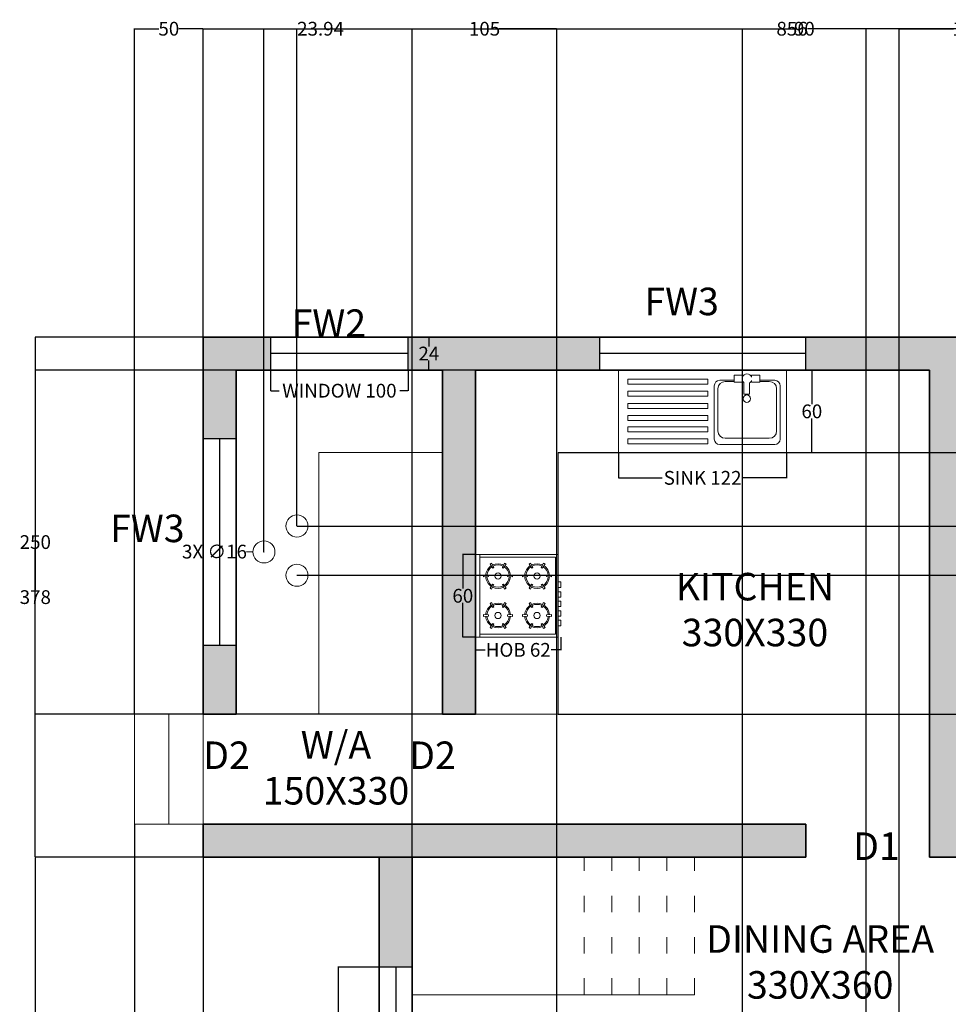
# Model space of a CAD drawing. Units: centimetres. Extents: x 1399 to 2860, y -110 to 1386.
# Tile 2 of 3: x 1399 to 2074, y 670 to 1386. Entities that reach past the tile are written whole.
import ezdxf

# ---------------------------------------------------------------- set-up
doc = ezdxf.new("R2010")
doc.units = ezdxf.units.CM
doc.header["$MEASUREMENT"] = 0
doc.linetypes.add('ACAD_ISO03W100', pattern=[30, 12, -18])
for name, color, linetype, lineweight in [('A-ANNO-DIMS', 2, 'Continuous', 18), ('A-ANNO-TEXT', 7, 'Continuous', 18), ('A-AREA-IDEN', 7, 'Continuous', 25), ('A-EQPM', 9, 'Continuous', 18), ('A-FLOR-CASE', 9, 'Continuous', 18), ('A-FLOR-FIXT', 9, 'Continuous', 18), ('A-FLOR-STRS', 7, 'Continuous', 18), ('A-FLOR-STRS-OVHD', 8, 'ACAD_ISO03W100', 18), ('A-GLAZ', 4, 'Continuous', 25), ('A-WALL', 7, 'Continuous', 35), ('A-WALL-PATT', 252, 'Continuous', 13)]:
    doc.layers.add(name, color=color, linetype=linetype, lineweight=lineweight)
doc.styles.get("Standard").update_dxf_attribs({"font": 'arial.ttf'})
doc.dimstyles.get("Standard").update_dxf_attribs({"dimtxt": 10, "dimasz": 0.18, "dimexe": 0.18, "dimexo": 0.0625, "dimgap": 0.09, "dimtad": 0, "dimtih": 1, "dimtoh": 1, "dimdec": 4, "dimzin": 0, "dimdsep": 46, "dimtxsty": 'Standard', "dimcen": 0.09, "dimadec": 0, "dimazin": 0, "dimtfac": 1, "dimtdec": 4, "dimtofl": 0, "dimtmove": 0, "dimatfit": 3, "dimfxl": 1, "dimtolj": 1, "dimtzin": 0, "dimarcsym": 0})

# ---------------------------------------------------------------- blocks, each defined once
blk = doc.blocks.new('w2')
blk.add_line((1776.97, 1807.89), (1676.97, 1807.89))
blk.add_lwpolyline([(1676.97, 1795.89), (1776.97, 1795.89), (1776.97, 1819.89), (1676.97, 1819.89)], close=True)
blk = doc.blocks.new('w3')
blk.add_line((1235.35, 1319.41), (1085.35, 1319.41))
blk.add_lwpolyline([(1085.35, 1307.41), (1235.35, 1307.41), (1235.35, 1331.41), (1085.35, 1331.41)], close=True)
blk = doc.blocks.new('A$C27DD639B')
for p, q in [((0, 0), (0, 450)), ((0, 450), (916.2, 450)), ((916.2, 0), (916.2, 450)), ((50.5, 372.3), (50.5, 400.1)), ((50.5, 400.1), (486.3, 400.1)), ((486.3, 400.1), (486.3, 372.3)), ((551.5, 394.1), (630.4, 394.1)), ((581.5, 388), (630.4, 388)), ((630.4, 383.4), (630.4, 422.8)), ((630.4, 422.8), (674.9, 422.8)), ((674.9, 383.4), (630.4, 383.4)), ((674.9, 422.8), (674.9, 411.1)), ((674.9, 394.1), (674.9, 383.4)), ((683, 318.7), (683, 382.1)), ((714.2, 379.9), (714.2, 318.7)), ((725.3, 411.7), (725.3, 422.8)), ((725.3, 422.8), (769.8, 422.8)), ((725.3, 383.4), (725.3, 393.5)), ((769.8, 383.4), (725.3, 383.4)), ((769.8, 422.8), (769.8, 383.4)), ((769.8, 394.1), (851.5, 394.1)), ((769.8, 388), (821.5, 388)), ((486.3, 372.3), (50.5, 372.3)), ((50.5, 307.4), (50.5, 335.2)), ((50.5, 335.2), (486.3, 335.2)), ((486.3, 335.2), (486.3, 307.4)), ((521.5, 74.1), (521.5, 364.1)), ((541.5, 118), (541.5, 348)), ((861.5, 348), (861.5, 118)), ((881.5, 364.1), (881.5, 74.1)), ((486.3, 307.4), (50.5, 307.4)), ((714.2, 318.7), (683, 318.7)), ((50.5, 240.3), (50.5, 268.1)), ((50.5, 268.1), (486.3, 268.1)), ((486.3, 240.3), (50.5, 240.3)), ((486.3, 268.1), (486.3, 240.3)), ((50.5, 175.4), (50.5, 203.2)), ((50.5, 203.2), (486.3, 203.2)), ((486.3, 175.4), (50.5, 175.4)), ((486.3, 203.2), (486.3, 175.4)), ((50.5, 112.8), (50.5, 140.6)), ((50.5, 140.6), (486.3, 140.6)), ((486.3, 112.8), (50.5, 112.8)), ((486.3, 140.6), (486.3, 112.8)), ((50.5, 48), (50.5, 75.8)), ((50.5, 75.8), (486.3, 75.8)), ((486.3, 75.8), (486.3, 48)), ((821.5, 78), (581.5, 78)), ((486.3, 48), (50.5, 48)), ((851.5, 44.1), (551.5, 44.1)), ((916.2, 0), (0, 0))]:
    blk.add_line(p, q)
blk.add_circle((699.5, 294.1), 20.1)
for centre, radius, start, end in [((700.2, 402.6), 26.7, 19.9093, 161.5199), ((551.5, 364.1), 30, 90, 180), ((581.5, 348), 40, 90, 180), ((700.2, 402.6), 26.7, 198.4801, 230.0288), ((700.2, 402.6), 26.7, 301.5638, 340.0907), ((821.5, 348), 40, 0, 90), ((851.5, 364.1), 30, 0, 90), ((581.5, 118), 40, 180, 270), ((821.5, 118), 40, 270, 0), ((551.5, 74.1), 30, 180, 270), ((851.5, 74.1), 30, 270, 0)]:
    blk.add_arc(centre, radius, start, end)
blk = doc.blocks.new('A$C756A3D80')
for p, q in [((600, 620), (0, 620)), ((0, 620), (0, 20)), ((0, 590), (600, 590)), ((20, 590), (20, 40)), ((580, 40), (580, 590)), ((600, 20), (600, 620)), ((69, 515.1), (62.3, 503.4)), ((62.3, 503.4), (94.8, 487.7)), ((98.8, 494.7), (69, 515.1)), ((163.4, 561.8), (149.9, 561.8)), ((149.9, 561.8), (152.6, 525.8)), ((152.6, 525.8), (160.7, 525.8)), ((160.7, 525.8), (163.4, 561.8)), ((244.3, 515.1), (214.5, 494.7)), ((218.6, 487.7), (251.1, 503.4)), ((251.1, 503.4), (244.3, 515.1)), ((355.7, 515.1), (348.9, 503.4)), ((348.9, 503.4), (381.4, 487.7)), ((385.5, 494.7), (355.7, 515.1)), ((450.1, 561.8), (436.6, 561.8)), ((436.6, 561.8), (439.3, 525.8)), ((439.3, 525.8), (447.4, 525.8)), ((447.4, 525.8), (450.1, 561.8)), ((531, 515.1), (501.2, 494.7)), ((505.2, 487.7), (537.7, 503.4)), ((537.7, 503.4), (531, 515.1)), ((94.8, 487.7), (98.8, 494.7)), ((214.5, 494.7), (218.6, 487.7)), ((381.4, 487.7), (385.5, 494.7)), ((501.2, 494.7), (505.2, 487.7)), ((94.8, 425.6), (62.3, 410)), ((62.3, 410), (69, 398.3)), ((69, 398.3), (98.8, 418.6)), ((98.8, 418.6), (94.8, 425.6)), ((152.6, 387.5), (149.9, 351.5)), ((160.7, 387.5), (152.6, 387.5)), ((163.4, 351.5), (160.7, 387.5)), ((218.6, 425.6), (214.5, 418.6)), ((214.5, 418.6), (244.3, 398.3)), ((251.1, 410), (218.6, 425.6)), ((244.3, 398.3), (251.1, 410)), ((381.4, 425.6), (348.9, 410)), ((348.9, 410), (355.7, 398.3)), ((355.7, 398.3), (385.5, 418.6)), ((385.5, 418.6), (381.4, 425.6)), ((439.3, 387.5), (436.6, 351.5)), ((447.4, 387.5), (439.3, 387.5)), ((450.1, 351.5), (447.4, 387.5)), ((505.2, 425.6), (501.2, 418.6)), ((501.2, 418.6), (531, 398.3)), ((537.7, 410), (505.2, 425.6)), ((531, 398.3), (537.7, 410)), ((149.9, 351.5), (163.4, 351.5)), ((436.6, 351.5), (450.1, 351.5)), ((69, 231.7), (62.3, 220)), ((62.3, 220), (94.8, 204.4)), ((98.8, 211.4), (69, 231.7)), ((163.4, 278.5), (149.9, 278.5)), ((149.9, 278.5), (152.6, 242.5)), ((152.6, 242.5), (160.7, 242.5)), ((160.7, 242.5), (163.4, 278.5)), ((244.3, 231.7), (214.5, 211.4)), ((218.6, 204.4), (251.1, 220)), ((251.1, 220), (244.3, 231.7)), ((355.7, 231.7), (348.9, 220)), ((348.9, 220), (381.4, 204.4)), ((385.5, 211.4), (355.7, 231.7)), ((450.1, 278.5), (436.6, 278.5)), ((436.6, 278.5), (439.3, 242.5)), ((439.3, 242.5), (447.4, 242.5)), ((447.4, 242.5), (450.1, 278.5)), ((531, 231.7), (501.2, 211.4)), ((505.2, 204.4), (537.7, 220)), ((537.7, 220), (531, 231.7)), ((94.8, 204.4), (98.8, 211.4)), ((214.5, 211.4), (218.6, 204.4)), ((381.4, 204.4), (385.5, 211.4)), ((501.2, 211.4), (505.2, 204.4)), ((94.8, 142.3), (62.3, 126.6)), ((62.3, 126.6), (69, 114.9)), ((69, 114.9), (98.8, 135.3)), ((98.8, 135.3), (94.8, 142.3)), ((152.6, 104.2), (149.9, 68.2)), ((160.7, 104.2), (152.6, 104.2)), ((163.4, 68.2), (160.7, 104.2)), ((218.6, 142.3), (214.5, 135.3)), ((214.5, 135.3), (244.3, 114.9)), ((251.1, 126.6), (218.6, 142.3)), ((244.3, 114.9), (251.1, 126.6)), ((381.4, 142.3), (348.9, 126.6)), ((348.9, 126.6), (355.7, 114.9)), ((355.7, 114.9), (385.5, 135.3)), ((385.5, 135.3), (381.4, 142.3)), ((439.3, 104.2), (436.6, 68.2)), ((447.4, 104.2), (439.3, 104.2)), ((450.1, 68.2), (447.4, 104.2)), ((505.2, 142.3), (501.2, 135.3)), ((501.2, 135.3), (531, 114.9)), ((537.7, 126.6), (505.2, 142.3)), ((531, 114.9), (537.7, 126.6)), ((0, 20), (600, 20)), ((20, 40), (580, 40)), ((81.8, 20), (121.8, 20)), ((81.8, 0), (81.8, 20)), ((121.8, 20), (121.8, 0)), ((149.9, 68.2), (163.4, 68.2)), ((151.3, 20), (191.3, 20)), ((151.3, 0), (151.3, 20)), ((191.3, 20), (191.3, 0)), ((221.6, 20), (261.6, 20)), ((221.6, 0), (221.6, 20)), ((261.6, 20), (261.6, 0)), ((289.3, 20), (329.3, 20)), ((289.3, 0), (289.3, 20)), ((329.3, 20), (329.3, 0)), ((361, 20), (401, 20)), ((361, 0), (361, 20)), ((401, 20), (401, 0)), ((436.6, 68.2), (450.1, 68.2)), ((121.8, 0), (81.8, 0)), ((191.3, 0), (151.3, 0)), ((261.6, 0), (221.6, 0)), ((329.3, 0), (289.3, 0)), ((401, 0), (361, 0))]:
    blk.add_line(p, q)
for centre in [(156.7, 456.7), (443.3, 456.7), (156.7, 173.3), (443.3, 173.3)]:
    blk.add_circle(centre, 22.6)
for centre, radius, start, end in [((156.7, 456.7), 90, 93.56902, 146.43098), ((156.7, 456.7), 81, 93.489, 146.511), ((156.7, 456.7), 81, 33.489, 86.511), ((156.7, 456.7), 90, 33.56902, 86.43098), ((443.3, 456.7), 90, 93.56902, 146.43098), ((443.3, 456.7), 81, 93.489, 146.511), ((443.3, 456.7), 81, 33.489, 86.511), ((443.3, 456.7), 90, 33.56902, 86.43098), ((156.7, 456.7), 90, 153.56902, 206.43098), ((156.7, 456.7), 81, 153.489, 206.511), ((156.7, 456.7), 81, 333.489, 26.511), ((156.7, 456.7), 90, 333.56902, 26.43098), ((443.3, 456.7), 90, 153.56902, 206.43098), ((443.3, 456.7), 81, 153.489, 206.511), ((443.3, 456.7), 81, 333.489, 26.511), ((443.3, 456.7), 90, 333.56902, 26.43098), ((156.7, 456.7), 90, 213.56902, 266.43098), ((156.7, 456.7), 81, 213.489, 266.511), ((156.7, 456.7), 81, 273.489, 326.511), ((156.7, 456.7), 90, 273.56902, 326.43098), ((443.3, 456.7), 90, 213.56902, 266.43098), ((443.3, 456.7), 81, 213.489, 266.511), ((443.3, 456.7), 81, 273.489, 326.511), ((443.3, 456.7), 90, 273.56902, 326.43098), ((156.7, 173.3), 90, 93.56902, 146.43098), ((156.7, 173.3), 81, 93.489, 146.511), ((156.7, 173.3), 81, 33.489, 86.511), ((156.7, 173.3), 90, 33.56902, 86.43098), ((443.3, 173.3), 90, 93.56902, 146.43098), ((443.3, 173.3), 81, 93.489, 146.511), ((443.3, 173.3), 81, 33.489, 86.511), ((443.3, 173.3), 90, 33.56902, 86.43098), ((156.7, 173.3), 90, 153.56902, 206.43098), ((156.7, 173.3), 81, 153.489, 206.511), ((156.7, 173.3), 81, 333.489, 26.511), ((156.7, 173.3), 90, 333.56902, 26.43098), ((443.3, 173.3), 90, 153.56902, 206.43098), ((443.3, 173.3), 81, 153.489, 206.511), ((443.3, 173.3), 81, 333.489, 26.511), ((443.3, 173.3), 90, 333.56902, 26.43098), ((156.7, 173.3), 90, 213.56902, 266.43098), ((156.7, 173.3), 81, 213.489, 266.511), ((156.7, 173.3), 81, 273.489, 326.511), ((156.7, 173.3), 90, 273.56902, 326.43098), ((443.3, 173.3), 90, 213.56902, 266.43098), ((443.3, 173.3), 81, 213.489, 266.511), ((443.3, 173.3), 81, 273.489, 326.511), ((443.3, 173.3), 90, 273.56902, 326.43098)]:
    blk.add_arc(centre, radius, start, end)
blk = doc.blocks.new('W4')
blk.add_line((1292.48, 2297.53), (1492.48, 2297.53))
blk.add_lwpolyline([(1292.48, 2285.53), (1492.48, 2285.53), (1492.48, 2309.53), (1292.48, 2309.53)], close=True)
blk = doc.blocks.new('*D19')
at = {"layer": 'A-ANNO-DIMS', "color": 0, "lineweight": -2, "transparency": 16777216}
for p, q in [((1581.8, 1130.95), (1581.8, 1115.83)), ((1681.8, 1130.95), (1681.8, 1115.83)), ((1581.98, 1116.01), (1587.89, 1116.01)), ((1681.62, 1116.01), (1675.72, 1116.01))]:
    blk.add_line(p, q, dxfattribs=at)
at = {"layer": 'A-ANNO-DIMS', "color": 0, "transparency": 16777216}
for points in [[(1581.98, 1116.04), (1581.98, 1115.98), (1581.8, 1116.01)], [(1681.62, 1116.04), (1681.62, 1115.98), (1681.8, 1116.01)]]:
    blk.add_solid(points, dxfattribs=at)
at = {"layer": 'Defpoints', "color": 0, "transparency": 16777216}
for p in [(1581.8, 1131.01), (1681.8, 1131.01), (1681.8, 1116.01)]:
    blk.add_point(p, dxfattribs=at)
at = {"layer": 'A-ANNO-DIMS', "color": 0, "transparency": 16777216, "insert": (1631.8, 1116.01), "char_height": 10, "attachment_point": 5}
blk.add_mtext('\\A1;WINDOW 100', dxfattribs=at)
blk = doc.blocks.new('*D20')
at = {"layer": 'A-ANNO-DIMS', "color": 0, "lineweight": -2, "transparency": 16777216}
for p, q in [((1681.86, 1155.01), (1696.98, 1155.01)), ((1696.8, 1154.83), (1696.8, 1148.12)), ((1696.8, 1131.19), (1696.8, 1137.9)), ((1681.86, 1131.01), (1696.98, 1131.01))]:
    blk.add_line(p, q, dxfattribs=at)
at = {"layer": 'A-ANNO-DIMS', "color": 0, "transparency": 16777216}
for points in [[(1696.77, 1154.83), (1696.83, 1154.83), (1696.8, 1155.01)], [(1696.77, 1131.19), (1696.83, 1131.19), (1696.8, 1131.01)]]:
    blk.add_solid(points, dxfattribs=at)
at = {"layer": 'Defpoints', "color": 0, "transparency": 16777216}
for p in [(1681.8, 1155.01), (1696.8, 1155.01), (1681.8, 1131.01)]:
    blk.add_point(p, dxfattribs=at)
at = {"layer": 'A-ANNO-DIMS', "color": 0, "transparency": 16777216, "insert": (1696.8, 1143.01), "char_height": 10, "attachment_point": 5}
blk.add_mtext('\\A1;24', dxfattribs=at)
blk = doc.blocks.new('*D21')
at = {"layer": 'A-ANNO-DIMS', "color": 0, "lineweight": -2, "transparency": 16777216}
for p, q in [((1660.74, 697.01), (1630.62, 697.01)), ((1630.8, 696.83), (1630.8, 602.27)), ((1630.8, 497.19), (1630.8, 591.75)), ((1660.74, 497.01), (1630.62, 497.01))]:
    blk.add_line(p, q, dxfattribs=at)
at = {"layer": 'A-ANNO-DIMS', "color": 0, "transparency": 16777216}
for points in [[(1630.77, 696.83), (1630.83, 696.83), (1630.8, 697.01)], [(1630.77, 497.19), (1630.83, 497.19), (1630.8, 497.01)]]:
    blk.add_solid(points, dxfattribs=at)
at = {"layer": 'Defpoints', "color": 0, "transparency": 16777216}
for p in [(1660.8, 697.01), (1630.8, 497.01), (1660.8, 497.01)]:
    blk.add_point(p, dxfattribs=at)
at = {"layer": 'A-ANNO-DIMS', "color": 0, "transparency": 16777216, "insert": (1630.8, 597.01), "char_height": 10, "attachment_point": 5}
blk.add_mtext('\\A1;WINDOW 200', dxfattribs=at)
blk = doc.blocks.new('*D33')
at = {"layer": 'A-ANNO-DIMS', "color": 0, "lineweight": -2, "transparency": 16777216}
for p, q in [((1834.73, 1070.95), (1834.73, 1052.51)), ((1956.88, 1070.95), (1956.88, 1052.51)), ((1834.91, 1052.69), (1866.5, 1052.69)), ((1956.7, 1052.69), (1925.11, 1052.69))]:
    blk.add_line(p, q, dxfattribs=at)
at = {"layer": 'A-ANNO-DIMS', "color": 0, "transparency": 16777216}
for points in [[(1834.91, 1052.72), (1834.91, 1052.66), (1834.73, 1052.69)], [(1956.7, 1052.72), (1956.7, 1052.66), (1956.88, 1052.69)]]:
    blk.add_solid(points, dxfattribs=at)
at = {"layer": 'Defpoints', "color": 0, "transparency": 16777216}
for p in [(1834.73, 1071.01), (1956.88, 1071.01), (1956.88, 1052.69)]:
    blk.add_point(p, dxfattribs=at)
at = {"layer": 'A-ANNO-DIMS', "color": 0, "transparency": 16777216, "insert": (1895.8, 1052.69), "char_height": 10, "attachment_point": 5}
blk.add_mtext('\\A1;SINK 122', dxfattribs=at)
blk = doc.blocks.new('*D34')
at = {"layer": 'A-ANNO-DIMS', "color": 0, "lineweight": -2, "transparency": 16777216}
for p, q in [((1956.94, 1131.01), (1975.38, 1131.01)), ((1975.2, 1130.83), (1975.2, 1106.21)), ((1975.2, 1071.19), (1975.2, 1095.81)), ((1956.94, 1071.01), (1975.38, 1071.01))]:
    blk.add_line(p, q, dxfattribs=at)
at = {"layer": 'A-ANNO-DIMS', "color": 0, "transparency": 16777216}
for points in [[(1975.17, 1130.83), (1975.23, 1130.83), (1975.2, 1131.01)], [(1975.17, 1071.19), (1975.23, 1071.19), (1975.2, 1071.01)]]:
    blk.add_solid(points, dxfattribs=at)
at = {"layer": 'Defpoints', "color": 0, "transparency": 16777216}
for p in [(1956.88, 1131.01), (1975.2, 1131.01), (1956.88, 1071.01)]:
    blk.add_point(p, dxfattribs=at)
at = {"layer": 'A-ANNO-DIMS', "color": 0, "transparency": 16777216, "insert": (1975.2, 1101.01), "char_height": 10, "attachment_point": 5}
blk.add_mtext('\\A1;60', dxfattribs=at)
blk = doc.blocks.new('*D35')
at = {"layer": 'A-ANNO-DIMS', "color": 0, "lineweight": -2, "transparency": 16777216}
for p, q in [((1730.8, 936.91), (1730.8, 927.5)), ((1792.8, 936.91), (1792.8, 927.5)), ((1730.98, 927.68), (1737.79, 927.68)), ((1792.62, 927.68), (1785.81, 927.68))]:
    blk.add_line(p, q, dxfattribs=at)
at = {"layer": 'A-ANNO-DIMS', "color": 0, "transparency": 16777216}
for points in [[(1730.98, 927.71), (1730.98, 927.65), (1730.8, 927.68)], [(1792.62, 927.71), (1792.62, 927.65), (1792.8, 927.68)]]:
    blk.add_solid(points, dxfattribs=at)
at = {"layer": 'Defpoints', "color": 0, "transparency": 16777216}
for p in [(1730.8, 936.98), (1792.8, 936.98), (1730.8, 927.68)]:
    blk.add_point(p, dxfattribs=at)
at = {"layer": 'A-ANNO-DIMS', "color": 0, "transparency": 16777216, "insert": (1761.8, 927.68), "char_height": 10, "attachment_point": 5}
blk.add_mtext('\\A1;HOB 62', dxfattribs=at)
blk = doc.blocks.new('*D36')
at = {"layer": 'A-ANNO-DIMS', "color": 0, "lineweight": -2, "transparency": 16777216}
for p, q in [((1730.74, 996.98), (1721.32, 996.98)), ((1721.5, 996.8), (1721.5, 972.17)), ((1721.5, 937.16), (1721.5, 961.78)), ((1730.74, 936.98), (1721.32, 936.98))]:
    blk.add_line(p, q, dxfattribs=at)
at = {"layer": 'A-ANNO-DIMS', "color": 0, "transparency": 16777216}
for points in [[(1721.47, 996.8), (1721.53, 996.8), (1721.5, 996.98)], [(1721.47, 937.16), (1721.53, 937.16), (1721.5, 936.98)]]:
    blk.add_solid(points, dxfattribs=at)
at = {"layer": 'Defpoints', "color": 0, "transparency": 16777216}
for p in [(1721.5, 996.98), (1730.8, 996.98), (1730.8, 936.98)]:
    blk.add_point(p, dxfattribs=at)
at = {"layer": 'A-ANNO-DIMS', "color": 0, "transparency": 16777216, "insert": (1721.5, 966.98), "char_height": 10, "attachment_point": 5}
blk.add_mtext('\\A1;60', dxfattribs=at)
blk = doc.blocks.new('*D37')
at = {"layer": 'A-ANNO-DIMS', "color": 0, "lineweight": -2, "transparency": 16777216}
for p, q in [((1482.8, 800.95), (1482.8, -103.22)), ((2766.8, -31.05), (2766.8, -103.22)), ((1482.98, -103.04), (2110.27, -103.04)), ((2766.62, -103.04), (2139.33, -103.04))]:
    blk.add_line(p, q, dxfattribs=at)
at = {"layer": 'A-ANNO-DIMS', "color": 0, "transparency": 16777216}
for points in [[(1482.98, -103.01), (1482.98, -103.07), (1482.8, -103.04)], [(2766.62, -103.01), (2766.62, -103.07), (2766.8, -103.04)]]:
    blk.add_solid(points, dxfattribs=at)
at = {"layer": 'Defpoints', "color": 0, "transparency": 16777216}
for p in [(1482.8, 801.01), (2766.8, -30.99), (2766.8, -103.04)]:
    blk.add_point(p, dxfattribs=at)
at = {"layer": 'A-ANNO-DIMS', "color": 0, "transparency": 16777216, "insert": (2124.8, -103.04), "char_height": 10, "attachment_point": 5}
blk.add_mtext('\\A1;1284', dxfattribs=at)
blk = doc.blocks.new('*D39')
at = {"layer": 'A-ANNO-DIMS', "color": 0, "lineweight": -2, "transparency": 16777216}
for p, q in [((1532.8, 1155.07), (1532.8, 1379.24)), ((1532.98, 1379.06), (1949.66, 1379.06)), ((2388.62, 1379.06), (1971.94, 1379.06)), ((2388.8, 1155.07), (2388.8, 1379.24))]:
    blk.add_line(p, q, dxfattribs=at)
at = {"layer": 'A-ANNO-DIMS', "color": 0, "transparency": 16777216}
for points in [[(1532.98, 1379.09), (1532.98, 1379.03), (1532.8, 1379.06)], [(2388.62, 1379.09), (2388.62, 1379.03), (2388.8, 1379.06)]]:
    blk.add_solid(points, dxfattribs=at)
at = {"layer": 'Defpoints', "color": 0, "transparency": 16777216}
for p in [(2388.8, 1379.06), (1532.8, 1155.01), (2388.8, 1155.01)]:
    blk.add_point(p, dxfattribs=at)
at = {"layer": 'A-ANNO-DIMS', "color": 0, "transparency": 16777216, "insert": (1960.8, 1379.06), "char_height": 10, "attachment_point": 5}
blk.add_mtext('\\A1;856', dxfattribs=at)
blk = doc.blocks.new('*D40')
at = {"layer": 'A-ANNO-DIMS', "color": 0, "lineweight": -2, "transparency": 16777216}
for p, q in [((1532.74, 1155.01), (1410.57, 1155.01)), ((1410.75, 1154.83), (1410.75, 971.21)), ((1410.75, 777.19), (1410.75, 960.81)), ((1532.74, 777.01), (1410.57, 777.01))]:
    blk.add_line(p, q, dxfattribs=at)
at = {"layer": 'A-ANNO-DIMS', "color": 0, "transparency": 16777216}
for points in [[(1410.72, 1154.83), (1410.78, 1154.83), (1410.75, 1155.01)], [(1410.72, 777.19), (1410.78, 777.19), (1410.75, 777.01)]]:
    blk.add_solid(points, dxfattribs=at)
at = {"layer": 'Defpoints', "color": 0, "transparency": 16777216}
for p in [(1410.75, 1155.01), (1532.8, 1155.01), (1532.8, 777.01)]:
    blk.add_point(p, dxfattribs=at)
at = {"layer": 'A-ANNO-DIMS', "color": 0, "transparency": 16777216, "insert": (1410.75, 966.01), "char_height": 10, "attachment_point": 5}
blk.add_mtext('\\A1;378', dxfattribs=at)
blk = doc.blocks.new('*D41')
at = {"layer": 'A-ANNO-DIMS', "color": 0, "lineweight": -2, "transparency": 16777216}
for p, q in [((1532.8, 776.95), (1532.8, -103.22)), ((1660.8, 776.95), (1660.8, -103.22)), ((1532.98, -103.04), (1586.13, -103.04)), ((1660.62, -103.04), (1607.48, -103.04))]:
    blk.add_line(p, q, dxfattribs=at)
at = {"layer": 'A-ANNO-DIMS', "color": 0, "transparency": 16777216}
for points in [[(1532.98, -103.01), (1532.98, -103.07), (1532.8, -103.04)], [(1660.62, -103.01), (1660.62, -103.07), (1660.8, -103.04)]]:
    blk.add_solid(points, dxfattribs=at)
at = {"layer": 'Defpoints', "color": 0, "transparency": 16777216}
for p in [(1532.8, 777.01), (1660.8, 777.01), (1660.8, -103.04)]:
    blk.add_point(p, dxfattribs=at)
at = {"layer": 'A-ANNO-DIMS', "color": 0, "transparency": 16777216, "insert": (1596.8, -103.04), "char_height": 10, "attachment_point": 5}
blk.add_mtext('\\A1;128', dxfattribs=at)
blk = doc.blocks.new('*D42')
at = {"layer": 'A-ANNO-DIMS', "color": 0, "lineweight": -2, "transparency": 16777216}
for p, q in [((1482.8, 881.07), (1482.8, 1379.24)), ((1482.98, 1379.06), (1500.57, 1379.06)), ((1532.62, 1379.06), (1515.04, 1379.06)), ((1532.8, 881.07), (1532.8, 1379.24))]:
    blk.add_line(p, q, dxfattribs=at)
at = {"layer": 'A-ANNO-DIMS', "color": 0, "transparency": 16777216}
for points in [[(1482.98, 1379.09), (1482.98, 1379.03), (1482.8, 1379.06)], [(1532.62, 1379.09), (1532.62, 1379.03), (1532.8, 1379.06)]]:
    blk.add_solid(points, dxfattribs=at)
at = {"layer": 'Defpoints', "color": 0, "transparency": 16777216}
for p in [(1532.8, 1379.06), (1482.8, 881.01), (1532.8, 881.01)]:
    blk.add_point(p, dxfattribs=at)
at = {"layer": 'A-ANNO-DIMS', "color": 0, "transparency": 16777216, "insert": (1507.8, 1379.06), "char_height": 10, "attachment_point": 5}
blk.add_mtext('\\A1;50', dxfattribs=at)
blk = doc.blocks.new('*D43')
at = {"layer": 'A-ANNO-DIMS', "color": 0, "lineweight": -2, "transparency": 16777216}
for p, q in [((1924.8, 417.07), (1924.8, 1379.24)), ((1924.98, 1379.06), (1962.57, 1379.06)), ((2014.62, 1379.06), (1977.04, 1379.06)), ((2014.8, 417.07), (2014.8, 1379.24))]:
    blk.add_line(p, q, dxfattribs=at)
at = {"layer": 'A-ANNO-DIMS', "color": 0, "transparency": 16777216}
for points in [[(1924.98, 1379.09), (1924.98, 1379.03), (1924.8, 1379.06)], [(2014.62, 1379.09), (2014.62, 1379.03), (2014.8, 1379.06)]]:
    blk.add_solid(points, dxfattribs=at)
at = {"layer": 'Defpoints', "color": 0, "transparency": 16777216}
for p in [(2014.8, 1379.06), (1924.8, 417.01), (2014.8, 417.01)]:
    blk.add_point(p, dxfattribs=at)
at = {"layer": 'A-ANNO-DIMS', "color": 0, "transparency": 16777216, "insert": (1969.8, 1379.06), "char_height": 10, "attachment_point": 5}
blk.add_mtext('\\A1;90', dxfattribs=at)
blk = doc.blocks.new('*D45')
at = {"layer": 'A-ANNO-DIMS', "color": 0, "lineweight": -2, "transparency": 16777216}
for p, q in [((2038.8, 33.07), (2038.8, 1379.24)), ((2038.98, 1379.06), (2078.15, 1379.06)), ((2138.62, 1379.06), (2099.45, 1379.06)), ((2138.8, 183.07), (2138.8, 1379.24))]:
    blk.add_line(p, q, dxfattribs=at)
at = {"layer": 'A-ANNO-DIMS', "color": 0, "transparency": 16777216}
for points in [[(2038.98, 1379.09), (2038.98, 1379.03), (2038.8, 1379.06)], [(2138.62, 1379.09), (2138.62, 1379.03), (2138.8, 1379.06)]]:
    blk.add_solid(points, dxfattribs=at)
at = {"layer": 'Defpoints', "color": 0, "transparency": 16777216}
for p in [(2038.8, 1379.06), (2138.8, 183.01), (2038.8, 33.01)]:
    blk.add_point(p, dxfattribs=at)
at = {"layer": 'A-ANNO-DIMS', "color": 0, "transparency": 16777216, "insert": (2088.8, 1379.06), "char_height": 10, "attachment_point": 5}
blk.add_mtext('\\A1;100', dxfattribs=at)
blk = doc.blocks.new('*D48')
at = {"layer": 'A-ANNO-DIMS', "color": 0, "lineweight": -2, "transparency": 16777216}
for p, q in [((1684.8, 417.07), (1684.8, 1379.24)), ((1684.98, 1379.06), (1726.6, 1379.06)), ((1789.62, 1379.06), (1748.01, 1379.06)), ((1789.8, 417.07), (1789.8, 1379.24))]:
    blk.add_line(p, q, dxfattribs=at)
at = {"layer": 'A-ANNO-DIMS', "color": 0, "transparency": 16777216}
for points in [[(1684.98, 1379.09), (1684.98, 1379.03), (1684.8, 1379.06)], [(1789.62, 1379.09), (1789.62, 1379.03), (1789.8, 1379.06)]]:
    blk.add_solid(points, dxfattribs=at)
at = {"layer": 'Defpoints', "color": 0, "transparency": 16777216}
for p in [(1789.8, 1379.06), (1684.8, 417.01), (1789.8, 417.01)]:
    blk.add_point(p, dxfattribs=at)
at = {"layer": 'A-ANNO-DIMS', "color": 0, "transparency": 16777216, "insert": (1737.3, 1379.06), "char_height": 10, "attachment_point": 5}
blk.add_mtext('\\A1;105', dxfattribs=at)
blk = doc.blocks.new('*D49')
at = {"layer": 'A-ANNO-DIMS', "color": 0, "lineweight": -2, "transparency": 16777216}
for p, q in [((1730.74, 1131.01), (1410.57, 1131.01)), ((1410.75, 1130.83), (1410.75, 1011.21)), ((1410.75, 881.19), (1410.75, 1000.81)), ((1730.74, 881.01), (1410.57, 881.01))]:
    blk.add_line(p, q, dxfattribs=at)
at = {"layer": 'A-ANNO-DIMS', "color": 0, "transparency": 16777216}
for points in [[(1410.72, 1130.83), (1410.78, 1130.83), (1410.75, 1131.01)], [(1410.72, 881.19), (1410.78, 881.19), (1410.75, 881.01)]]:
    blk.add_solid(points, dxfattribs=at)
at = {"layer": 'Defpoints', "color": 0, "transparency": 16777216}
for p in [(1410.75, 1131.01), (1730.8, 1131.01), (1730.8, 881.01)]:
    blk.add_point(p, dxfattribs=at)
at = {"layer": 'A-ANNO-DIMS', "color": 0, "transparency": 16777216, "insert": (1410.75, 1006.01), "char_height": 10, "attachment_point": 5}
blk.add_mtext('\\A1;250', dxfattribs=at)
blk = doc.blocks.new('*D50')
at = {"layer": 'A-ANNO-DIMS', "color": 0, "lineweight": -2, "transparency": 16777216}
for p, q in [((1660.74, 777.01), (1410.57, 777.01)), ((1410.75, 776.83), (1410.75, 398.21)), ((1410.75, 9.19), (1410.75, 387.81)), ((1660.74, 9.01), (1410.57, 9.01))]:
    blk.add_line(p, q, dxfattribs=at)
at = {"layer": 'A-ANNO-DIMS', "color": 0, "transparency": 16777216}
for points in [[(1410.72, 776.83), (1410.78, 776.83), (1410.75, 777.01)], [(1410.72, 9.19), (1410.78, 9.19), (1410.75, 9.01)]]:
    blk.add_solid(points, dxfattribs=at)
at = {"layer": 'Defpoints', "color": 0, "transparency": 16777216}
for p in [(1410.75, 777.01), (1660.8, 777.01), (1660.8, 9.01)]:
    blk.add_point(p, dxfattribs=at)
at = {"layer": 'A-ANNO-DIMS', "color": 0, "transparency": 16777216, "insert": (1410.75, 393.01), "char_height": 10, "attachment_point": 5}
blk.add_mtext('\\A1;768', dxfattribs=at)
blk = doc.blocks.new('*D51')
at = {"layer": 'A-ANNO-DIMS', "color": 0, "lineweight": -2, "transparency": 16777216}
for p, q in [((1600.97, 1017.69), (2839.03, 1017.69)), ((2838.85, 1017.51), (2838.85, 1004.98)), ((2838.85, 982.05), (2838.85, 994.58)), ((1600.97, 981.87), (2839.03, 981.87))]:
    blk.add_line(p, q, dxfattribs=at)
at = {"layer": 'A-ANNO-DIMS', "color": 0, "transparency": 16777216}
for points in [[(2838.82, 1017.51), (2838.88, 1017.51), (2838.85, 1017.69)], [(2838.82, 982.05), (2838.88, 982.05), (2838.85, 981.87)]]:
    blk.add_solid(points, dxfattribs=at)
at = {"layer": 'Defpoints', "color": 0, "transparency": 16777216}
for p in [(1600.91, 1017.69), (1600.91, 981.87), (2838.85, 981.87)]:
    blk.add_point(p, dxfattribs=at)
at = {"layer": 'A-ANNO-DIMS', "color": 0, "transparency": 16777216, "insert": (2838.85, 999.78), "char_height": 10, "attachment_point": 5}
blk.add_mtext('\\A1;35.824', dxfattribs=at)
blk = doc.blocks.new('*D52')
at = {"layer": 'A-ANNO-DIMS', "color": 0, "lineweight": -2, "transparency": 16777216}
for p, q in [((1576.97, 998.94), (1576.97, 1379.24)), ((1577.15, 1379.06), (1600.73, 1379.06)), ((1600.91, 1017.75), (1600.91, 1379.24)), ((1600.91, 1379.06), (1601.09, 1379.06))]:
    blk.add_line(p, q, dxfattribs=at)
at = {"layer": 'A-ANNO-DIMS', "color": 0, "transparency": 16777216}
for points in [[(1577.15, 1379.09), (1577.15, 1379.03), (1576.97, 1379.06)], [(1600.73, 1379.09), (1600.73, 1379.03), (1600.91, 1379.06)]]:
    blk.add_solid(points, dxfattribs=at)
at = {"layer": 'Defpoints', "color": 0, "transparency": 16777216}
for p in [(1600.91, 1379.06), (1600.91, 1017.69), (1576.97, 998.88)]:
    blk.add_point(p, dxfattribs=at)
at = {"layer": 'A-ANNO-DIMS', "color": 0, "transparency": 16777216, "insert": (1618.11, 1379.06), "char_height": 10, "attachment_point": 5}
blk.add_mtext('\\A1;23.94', dxfattribs=at)
blk = doc.blocks.new('*D53')
at = {"layer": 'A-ANNO-DIMS', "color": 0, "lineweight": -2, "transparency": 16777216}
for p, q in [((1790.86, 1071.01), (2839.03, 1071.01)), ((2838.85, 1070.83), (2838.85, 981.21)), ((2838.85, 881.19), (2838.85, 970.81)), ((1790.86, 881.01), (2839.03, 881.01))]:
    blk.add_line(p, q, dxfattribs=at)
at = {"layer": 'A-ANNO-DIMS', "color": 0, "transparency": 16777216}
for points in [[(2838.82, 1070.83), (2838.88, 1070.83), (2838.85, 1071.01)], [(2838.82, 881.19), (2838.88, 881.19), (2838.85, 881.01)]]:
    blk.add_solid(points, dxfattribs=at)
at = {"layer": 'Defpoints', "color": 0, "transparency": 16777216}
for p in [(1790.8, 1071.01), (2838.85, 1071.01), (1790.8, 881.01)]:
    blk.add_point(p, dxfattribs=at)
at = {"layer": 'A-ANNO-DIMS', "color": 0, "transparency": 16777216, "insert": (2838.85, 976.01), "char_height": 10, "attachment_point": 5}
blk.add_mtext('\\A1;190', dxfattribs=at)
blk = doc.blocks.new('*D54')
at = {"layer": 'A-ANNO-DIMS', "color": 0, "lineweight": -2, "transparency": 16777216}
for p, q in [((1564.17, 999.08), (1568.79, 999)), ((1576.88, 998.88), (1577.06, 998.88)), ((1576.97, 998.79), (1576.97, 998.97))]:
    blk.add_line(p, q, dxfattribs=at)
at = {"layer": 'A-ANNO-DIMS', "color": 0, "transparency": 16777216}
blk.add_solid([(1568.79, 999.03), (1568.79, 998.97), (1568.97, 999)], dxfattribs=at)
at = {"layer": 'Defpoints', "color": 0, "transparency": 16777216}
for p in [(1568.97, 999), (1584.96, 998.75)]:
    blk.add_point(p, dxfattribs=at)
at = {"layer": 'A-ANNO-DIMS', "color": 0, "transparency": 16777216, "insert": (1541, 999.08), "char_height": 10, "attachment_point": 5}
blk.add_mtext('\\A1;3X ∅16', dxfattribs=at)

msp = doc.modelspace()

# ---------------------------------------------------------------- hatches: boundary and pattern name
at = {"layer": 'A-WALL-PATT'}
h = msp.add_hatch(color=256, dxfattribs=at)
h.dxf.hatch_style = 1
h.paths.add_polyline_path([(1581.8022, 1155.0098), (1532.8022, 1155.0098), (1532.8022, 1081.0098), (1556.8022, 1081.0098), (1556.8022, 1131.0098), (1581.8022, 1131.0098)])
h.paths.add_polyline_path([(1556.8022, 931.0098), (1532.8022, 931.0098), (1532.8022, 881.0098), (1556.8022, 881.0098)])
h.paths.add_polyline_path([(1820.8022, 1155.0098), (1681.8022, 1155.0098), (1681.8022, 1131.0098), (1706.8022, 1131.0098), (1706.8022, 881.0098), (1730.8022, 881.0098), (1730.8022, 1131.0098), (1820.8022, 1131.0098)])
h.paths.add_polyline_path([(2119.8022, 1155.0098), (1970.8022, 1155.0098), (1970.8022, 1131.0098), (2060.8022, 1131.0098), (2060.8022, 777.0098), (2084.8022, 777.0098), (2084.8022, 907.0098), (2134.8022, 907.0098), (2134.8022, 931.0098), (2084.8022, 931.0098), (2084.8022, 1131.0098), (2119.8022, 1131.0098)])
h.paths.add_polyline_path([(2283.8022, 1155.0098), (2179.8022, 1155.0098), (2179.8022, 1131.0098), (2214.8022, 1131.0098), (2214.8022, 907.0098), (2388.8022, 907.0098), (2388.8022, 857.0098), (2412.8022, 857.0098), (2412.8022, 931.0098), (2238.8022, 931.0098), (2238.8022, 1131.0098), (2283.8022, 1131.0098)])
h.paths.add_polyline_path([(2388.8022, 1155.0098), (2343.8022, 1155.0098), (2343.8022, 1131.0098), (2388.8022, 1131.0098)], flags=17)
h.paths.add_polyline_path([(2412.8022, 1283.0098), (2442.8022, 1283.0098), (2442.8022, 1307.0098), (2388.8022, 1307.0098), (2388.8022, 1011.0098), (2412.8022, 1011.0098)])
h.paths.add_polyline_path([(2662.8022, 1307.0098), (2492.8022, 1307.0098), (2492.8022, 1283.0098), (2662.8022, 1283.0098)])
h.paths.add_polyline_path([(2766.8022, 1307.0098), (2712.8022, 1307.0098), (2712.8022, 1283.0098), (2742.8022, 1283.0098), (2742.8022, 1157.0098), (2766.8022, 1157.0098)])
h.paths.add_polyline_path([(2766.8022, 1007.0098), (2742.8022, 1007.0098), (2742.8022, 881.0098), (2502.8022, 881.0098), (2502.8022, 717.0098), (2388.8022, 717.0098), (2388.8022, 693.0098), (2526.8022, 693.0098), (2526.8022, 857.0098), (2742.8022, 857.0098), (2742.8022, 817.0098), (2766.8022, 817.0098)])
h.paths.add_polyline_path([(2766.8022, 757.0098), (2742.8022, 757.0098), (2742.8022, 717.0098), (2606.8022, 717.0098), (2606.8022, 693.0098), (2742.8022, 693.0098), (2742.8022, 598.0098), (2766.8022, 598.0098)])
h.paths.add_polyline_path([(2442.8022, 353.0098), (2412.8022, 353.0098), (2412.8022, 603.0098), (2238.8022, 603.0098), (2238.8022, 579.0098), (2388.8022, 579.0098), (2388.8022, 512.2445, -0.02916898), (2388.8858, 510.8126), (2388.8858, 458.2748), (2388.8022, 458.2748), (2388.8022, 402.9002), (2388.8024, 402.776), (2388.8858, 402.776), (2388.8858, 350.2798, -0.02916898), (2388.8022, 348.8479), (2388.8022, 329.0098), (2442.8022, 329.0098)])
h.paths.add_polyline_path([(2662.8022, 353.0098), (2492.8022, 353.0098), (2492.8022, 329.0098), (2662.8022, 329.0098)])
h.paths.add_polyline_path([(2412.8022, 329.0098), (2388.8022, 329.0098), (2388.8022, 159.0098), (2412.8022, 159.0098)])
h.paths.add_polyline_path([(2388.8022, 183.0098), (2338.8022, 183.0098), (2338.8022, 159.0098), (2388.8022, 159.0098)])
h.paths.add_polyline_path([(2188.8022, 183.0098), (2138.8022, 183.0098), (2138.8022, 159.0098), (2188.8022, 159.0098)])
h.paths.add_polyline_path([(2038.8022, 417.0098), (2014.8022, 417.0098), (2014.8022, 33.0098), (1924.8022, 33.0098), (1924.8022, 9.0098), (2038.8022, 9.0098)])
h.paths.add_polyline_path([(1774.8022, 33.0098), (1684.8022, 33.0098), (1684.8022, 63.0098), (1660.8022, 63.0098), (1660.8022, 9.0098), (1774.8022, 9.0098)])
h.paths.add_polyline_path([(1684.8022, 313.0098), (1660.8022, 313.0098), (1660.8022, 113.0098), (1684.8022, 113.0098)])
h.paths.add_polyline_path([(1924.8022, 417.0098), (1684.8022, 417.0098), (1684.8022, 497.0098), (1660.8022, 497.0098), (1660.8022, 363.0098), (1684.8022, 363.0098), (1684.8022, 393.0098), (1924.8022, 393.0098)])
h.paths.add_polyline_path([(1684.8022, 777.0098), (1660.8022, 777.0098), (1660.8022, 697.0098), (1684.8022, 697.0098)])
h.paths.add_polyline_path([(1970.8022, 801.0098), (1532.8022, 801.0098), (1532.8022, 777.0098), (1970.8022, 777.0098)])

# ---------------------------------------------------------------- linework, layer by layer
at = {"layer": 'A-EQPM'}
for centre in [(1600.9054, 1017.6901), (1576.9658, 998.8751), (1600.9054, 981.8663)]:
    msp.add_circle(centre, 8, dxfattribs=at)
at = {"layer": 'A-FLOR-CASE'}
for p, q in [((1616.8022, 881.0098), (1616.8022, 1071.0098)), ((1616.8022, 1071.0098), (1706.8022, 1071.0098)), ((1790.8022, 881.0098), (1790.8022, 1071.0098)), ((1790.8022, 1071.0098), (2060.8022, 1071.0098)), ((1556.8022, 881.0098), (1616.8022, 881.0098)), ((1790.8022, 881.0098), (1730.8022, 881.0098))]:
    msp.add_line(p, q, dxfattribs=at)
at = {"layer": 'A-FLOR-STRS'}
for p, q in [((1482.8022, 881.0098), (1482.8022, 801.0098)), ((1532.8022, 881.0098), (1482.8022, 881.0098)), ((1507.8022, 881.0098), (1507.8022, 801.0098)), ((1532.8022, 881.0098), (1532.8022, 801.0098)), ((1532.8022, 801.0098), (1482.8022, 801.0098)), ((1789.8022, 677.0098), (1789.8022, 777.0098)), ((1684.8022, 677.0098), (1889.8022, 677.0098)), ((1789.8022, 417.0098), (1789.8022, 677.0098))]:
    msp.add_line(p, q, dxfattribs=at)
at = {"layer": 'A-FLOR-STRS-OVHD'}
for p, q in [((1809.8022, 677.0098), (1809.8022, 777.0098)), ((1829.8022, 677.0098), (1829.8022, 777.0098)), ((1849.8022, 677.0098), (1849.8022, 777.0098)), ((1869.8022, 677.0098), (1869.8022, 777.0098)), ((1889.8022, 677.0098), (1889.8022, 777.0098))]:
    msp.add_line(p, q, dxfattribs=at)
at = {"layer": 'A-WALL'}
for p, q in [((1532.8022, 1155.0098), (2388.8022, 1155.0098)), ((1532.8022, 881.0098), (1532.8022, 1155.0098)), ((1556.8022, 1131.0098), (1706.8022, 1131.0098)), ((1556.8022, 881.0098), (1556.8022, 1131.0098)), ((1706.8022, 881.0098), (1706.8022, 1131.0098)), ((1730.8022, 881.0098), (1730.8022, 1131.0098)), ((1730.8022, 1131.0098), (2060.8022, 1131.0098)), ((2060.8022, 777.0098), (2060.8022, 1131.0098)), ((1532.8022, 881.0098), (1556.8022, 881.0098)), ((1706.8022, 881.0098), (1730.8022, 881.0098)), ((1532.8022, 801.0098), (1970.8022, 801.0098)), ((1532.8022, 777.0098), (1532.8022, 801.0098)), ((1970.8022, 777.0098), (1970.8022, 801.0098)), ((1532.8022, 777.0098), (1970.8022, 777.0098)), ((1660.8022, 9.0098), (1660.8022, 777.0098)), ((1684.8022, 417.0098), (1684.8022, 777.0098)), ((2060.8022, 777.0098), (2084.8022, 777.0098))]:
    msp.add_line(p, q, dxfattribs=at)

# ---------------------------------------------------------------- block references
at = {"layer": 'A-EQPM', "xscale": 0.1, "yscale": 0.1, "zscale": 0.1, "rotation": 90}
msp.add_blockref('A$C756A3D80', (1792.8022, 936.9772), dxfattribs=at)
at = {"layer": 'A-FLOR-FIXT', "xscale": 0.1333333333333333, "yscale": 0.1333333333333333, "zscale": 0.1333333333333333}
msp.add_blockref('A$C27DD639B', (1834.7254, 1071.0098), dxfattribs=at)
at = {"layer": 'A-GLAZ'}
for name, p in [('w2', (-95.1654, -664.8776)), ('w3', (735.4552, -176.4003))]:
    msp.add_blockref(name, p, dxfattribs=at)
at = {"layer": 'A-GLAZ', "rotation": 270}
for name, p in [('w3', (225.392, 2166.3567)), ('W4', (-624.7289, 1989.489))]:
    msp.add_blockref(name, p, dxfattribs=at)

# ---------------------------------------------------------------- texts
at = {"layer": 'A-ANNO-TEXT', "char_height": 20, "attachment_point": 1}
for s, width, insert in [('FW3', 163.588182, (1853.4944, 1190.868)), ('FW2', 163.588182, (1597.0194, 1175.0917)), ('FW3', 163.588182, (1465.1019, 1025.955)), ('D2', 163.588182, (1532.8022, 861.0917)), ('D2', 163.588182, (1682.5201, 861.0917)), ('D1', 103.726959, (2005.2392, 795.0107))]:
    msp.add_mtext_dynamic_manual_height_columns(s, width=width, gutter_width=1, heights=[0], dxfattribs=dict(at, insert=insert))
at = {"layer": 'A-AREA-IDEN', "char_height": 20, "attachment_point": 1}
for s, insert in [('\\pxqc;KITCHEN\\P330X330', (1700.4943, 983.6109)), ('\\pxqc;W/A\\P150X330', (1395.9909, 868.6261)), ('\\pxqc;DINING AREA\\P330X360', (1747.9315, 727.5486))]:
    msp.add_mtext_dynamic_manual_height_columns(s, width=466.660539, gutter_width=1, heights=[0], dxfattribs=dict(at, insert=insert))

# ---------------------------------------------------------------- dimensions: what is measured, and where the dimension line sits
at = {"layer": 'A-ANNO-DIMS'}
for base, p1, p2, override, picture, middle in [((1532.8022, 1379.0598), (1482.8022, 881.0098), (1532.8022, 881.0098), {"dimdec": 0, "dimlfac": 1, "dimrnd": 0, "dimzin": 0, "dimdsep": 46, "dimlunit": 2}, '*D42', (1507.8022, 1379.0598)), ((2388.8022, 1379.0598), (1532.8022, 1155.0098), (2388.8022, 1155.0098), {"dimdec": 0, "dimlfac": 1, "dimrnd": 0, "dimzin": 0, "dimdsep": 46, "dimlunit": 2}, '*D39', (1960.8022, 1379.0598)), ((1600.9054, 1379.0598), (1576.9658, 998.8751), (1600.9054, 1017.6901), {"dimdec": 2, "dimlfac": 1, "dimrnd": 0, "dimzin": 0, "dimdsep": 46, "dimlunit": 2}, '*D52', (1618.1126, 1379.0598)), ((1789.8022, 1379.0598), (1684.8022, 417.0098), (1789.8022, 417.0098), {"dimdec": 0, "dimlfac": 1, "dimrnd": 0, "dimzin": 0, "dimdsep": 46, "dimlunit": 2}, '*D48', (1737.3022, 1379.0598)), ((2014.8022, 1379.0598), (1924.8022, 417.0098), (2014.8022, 417.0098), {"dimdec": 0, "dimlfac": 1, "dimrnd": 0, "dimzin": 0, "dimdsep": 46, "dimlunit": 2}, '*D43', (1969.8022, 1379.0598)), ((2038.8022, 1379.0598), (2138.8022, 183.0098), (2038.8022, 33.0098), {"dimdec": 0, "dimlfac": 1, "dimrnd": 0, "dimzin": 0, "dimdsep": 46, "dimlunit": 2}, '*D45', (2088.8022, 1379.0598)), ((2766.8022, -103.0402), (1482.8022, 801.0098), (2766.8022, -30.9902), {"dimdec": 0, "dimlfac": 1, "dimrnd": 0, "dimzin": 0, "dimdsep": 46, "dimlunit": 2}, '*D37', (2124.8022, -103.0402)), ((1660.8022, -103.0402), (1532.8022, 777.0098), (1660.8022, 777.0098), {"dimdec": 0, "dimlfac": 1, "dimrnd": 0, "dimzin": 0, "dimdsep": 46, "dimlunit": 2}, '*D41', (1596.8022, -103.0402))]:
    dim = msp.add_linear_dim(base=base, p1=p1, p2=p2, dimstyle='Standard', override=override, dxfattribs=at)
    dim.commit()
    dim.dimension.update_dxf_attribs({"geometry": picture, "text_midpoint": middle})
for base, p1, p2, override, picture, middle in [((1410.7522, 1155.0098), (1532.8022, 777.0098), (1532.8022, 1155.0098), {"dimdec": 0, "dimlfac": 1, "dimrnd": 0, "dimzin": 0, "dimdsep": 46, "dimlunit": 2}, '*D40', (1410.7522, 966.0098)), ((1696.8022, 1155.0098), (1681.8022, 1131.0098), (1681.8022, 1155.0098), {"dimdec": 0, "dimlfac": 1, "dimrnd": 0, "dimzin": 0, "dimdsep": 46, "dimlunit": 2}, '*D20', (1696.8022, 1143.0098)), ((1410.7522, 1131.0098), (1730.8022, 881.0098), (1730.8022, 1131.0098), {"dimdec": 0, "dimlfac": 1, "dimrnd": 0, "dimzin": 0, "dimdsep": 46, "dimlunit": 2}, '*D49', (1410.7522, 1006.0098)), ((1975.202, 1131.0098), (1956.8789, 1071.0098), (1956.8789, 1131.0098), {"dimdec": 0, "dimlfac": 1, "dimrnd": 0, "dimzin": 0, "dimdsep": 46, "dimlunit": 2}, '*D34', (1975.202, 1101.0098)), ((2838.8522, 1071.0098), (1790.8022, 881.0098), (1790.8022, 1071.0098), {"dimdec": 0, "dimlfac": 1, "dimrnd": 0, "dimzin": 0, "dimdsep": 46, "dimlunit": 2}, '*D53', (2838.8522, 976.0098)), ((2838.8522, 981.8663), (1600.9054, 1017.6901), (1600.9054, 981.8663), {"dimdec": 3, "dimlfac": 1, "dimrnd": 0, "dimzin": 0, "dimdsep": 46, "dimlunit": 2}, '*D51', (2838.8522, 999.7782)), ((1721.5022, 996.9772), (1730.8022, 936.9772), (1730.8022, 996.9772), {"dimdec": 0, "dimlfac": 1, "dimrnd": 0, "dimzin": 0, "dimdsep": 46, "dimlunit": 2}, '*D36', (1721.5022, 966.9772)), ((1410.7522, 777.0098), (1660.8022, 9.0098), (1660.8022, 777.0098), {"dimdec": 0, "dimlfac": 1, "dimrnd": 0, "dimzin": 0, "dimdsep": 46, "dimlunit": 2}, '*D50', (1410.7522, 393.0098))]:
    dim = msp.add_linear_dim(base=base, p1=p1, p2=p2, angle=90, dimstyle='Standard', override=override, dxfattribs=at)
    dim.commit()
    dim.dimension.update_dxf_attribs({"geometry": picture, "text_midpoint": middle})
for base, p1, p2, text, picture, middle in [((1681.8022, 1116.0098), (1581.8022, 1131.0098), (1681.8022, 1131.0098), 'WINDOW <>', '*D19', (1631.8022, 1116.0098)), ((1956.8789, 1052.6868), (1834.7254, 1071.0098), (1956.8789, 1071.0098), 'SINK <>', '*D33', (1895.8022, 1052.6868))]:
    dim = msp.add_linear_dim(base=base, p1=p1, p2=p2, text=text, dimstyle='Standard', override={"dimdec": 0, "dimlfac": 1, "dimrnd": 0, "dimzin": 0, "dimdsep": 46, "dimlunit": 2}, dxfattribs=at)
    dim.commit()
    dim.dimension.update_dxf_attribs({"geometry": picture, "text_midpoint": middle})
dim = msp.add_diameter_dim_2p(p1=(1584.9648, 998.7497), p2=(1568.9667, 999.0005), text='3X <>', dimstyle='Standard', override={"dimdec": 0, "dimlfac": 1, "dimrnd": 0, "dimzin": 0, "dimdsep": 46, "dimlunit": 2}, dxfattribs=at)
dim.commit()
dim.dimension.update_dxf_attribs({"geometry": '*D54', "text_midpoint": (1564.1673, 999.0758), "dimtype": 163})
for base, p1, p2, angle, text, picture, middle in [((1730.8022, 927.6772), (1792.8022, 936.9772), (1730.8022, 936.9772), 180, 'HOB <>', '*D35', (1761.8022, 927.6772)), ((1630.8022, 497.0098), (1660.8022, 697.0098), (1660.8022, 497.0098), 270, 'WINDOW <>', '*D21', (1630.8022, 597.0098))]:
    dim = msp.add_linear_dim(base=base, p1=p1, p2=p2, angle=angle, text=text, dimstyle='Standard', override={"dimdec": 0, "dimlfac": 1, "dimrnd": 0, "dimzin": 0, "dimdsep": 46, "dimlunit": 2}, dxfattribs=at)
    dim.commit()
    dim.dimension.update_dxf_attribs({"geometry": picture, "text_midpoint": middle})

doc.saveas('drawing.dxf')
